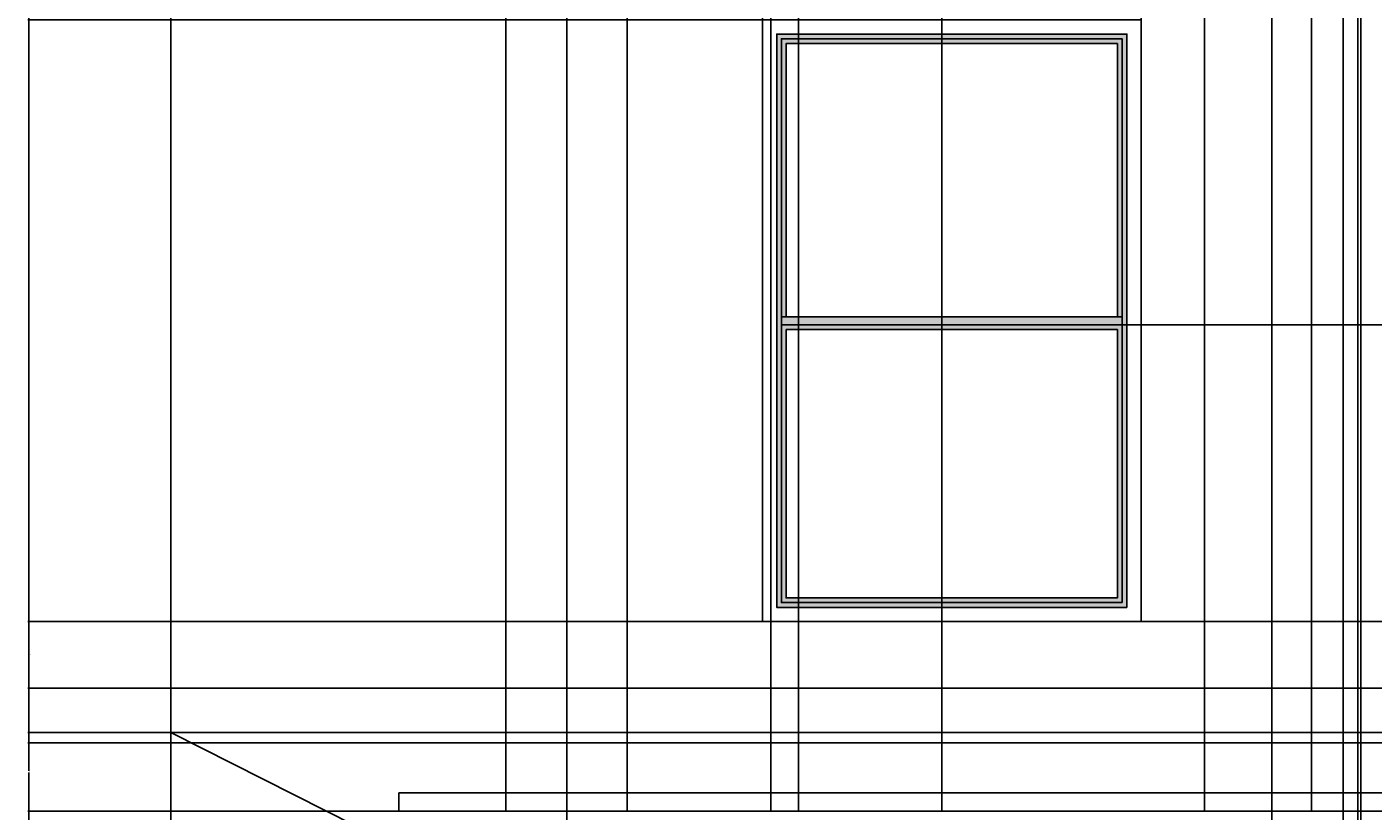
# Model space of a CAD drawing. Units: millimetres. Extents: x 171 to 1599, y 973 to 1509.
# Tile 3 of 7: x 951 to 1235, y 1178 to 1343. Entities that reach past the tile are written whole.
import ezdxf

# ---------------------------------------------------------------- set-up
doc = ezdxf.new("R2010")
doc.units = ezdxf.units.MM
for name, color, linetype, lineweight in [('A-ANNO-DIMS', 2, 'Continuous', 18), ('A-ELEV', 7, 'Continuous', 25), ('A-ELEV-FILL', 252, 'Continuous', 13)]:
    doc.layers.add(name, color=color, linetype=linetype, lineweight=lineweight)
doc.styles.get("Standard").update_dxf_attribs({"font": 'arial.ttf'})
doc.dimstyles.get("Standard").update_dxf_attribs({"dimtxt": 0.18, "dimasz": 0.18, "dimexe": 0.18, "dimexo": 0.0625, "dimgap": 0.09, "dimtad": 0, "dimtih": 1, "dimtoh": 1, "dimdec": 1, "dimzin": 0, "dimdsep": 46, "dimlunit": 3, "dimtxsty": 'Standard', "dimcen": 0.09, "dimadec": 0, "dimazin": 0, "dimtfac": 1, "dimtdec": 1, "dimtofl": 0, "dimtmove": 0, "dimatfit": 3, "dimfxl": 1, "dimtolj": 1, "dimtzin": 0, "dimarcsym": 0})

# ---------------------------------------------------------------- blocks, each defined once
blk = doc.blocks.new('*D1')
at = {"layer": 'A-ANNO-DIMS', "color": 0, "lineweight": -2, "transparency": 16777216}
for p, q in [((980.93, 1194.55), (980.93, 1508.31)), ((981.11, 1508.13), (1274.61, 1508.13)), ((1568.85, 1508.13), (1275.36, 1508.13)), ((1569.03, 1215.31), (1569.03, 1508.31))]:
    blk.add_line(p, q, dxfattribs=at)
at = {"layer": 'A-ANNO-DIMS', "color": 0, "transparency": 16777216}
for points in [[(981.11, 1508.16), (981.11, 1508.1), (980.93, 1508.13)], [(1568.85, 1508.16), (1568.85, 1508.1), (1569.03, 1508.13)]]:
    blk.add_solid(points, dxfattribs=at)
at = {"layer": 'Defpoints', "color": 0, "transparency": 16777216}
for p in [(1569.03, 1508.13), (1569.03, 1215.25), (980.93, 1194.49)]:
    blk.add_point(p, dxfattribs=at)
at = {"layer": 'A-ANNO-DIMS', "color": 0, "transparency": 16777216, "insert": (1274.98, 1508.13), "char_height": 0.18, "attachment_point": 5}
blk.add_mtext('\\A1;588.1', dxfattribs=at)
blk = doc.blocks.new('*D2')
at = {"layer": 'A-ANNO-DIMS', "color": 0, "lineweight": -2, "transparency": 16777216}
for p, q in [((1043.70287, 1478.130098), (1599.212656, 1478.130098)), ((1599.032656, 1477.950098), (1599.032656, 1240.959874)), ((1599.032656, 1003.60965), (1599.032656, 1240.599874)), ((1348.449149, 1003.42965), (1599.212656, 1003.42965))]:
    blk.add_line(p, q, dxfattribs=at)
at = {"layer": 'A-ANNO-DIMS', "color": 0, "transparency": 16777216}
for points in [[(1599.002656, 1477.950098), (1599.062656, 1477.950098), (1599.032656, 1478.130098)], [(1599.002656, 1003.60965), (1599.062656, 1003.60965), (1599.032656, 1003.42965)]]:
    blk.add_solid(points, dxfattribs=at)
at = {"layer": 'Defpoints', "color": 0, "transparency": 16777216}
for p in [(1043.64037, 1478.130098), (1599.032656, 1478.130098), (1348.386649, 1003.42965)]:
    blk.add_point(p, dxfattribs=at)
at = {"layer": 'A-ANNO-DIMS', "color": 0, "transparency": 16777216, "insert": (1599.032656, 1240.779874), "char_height": 0.18, "attachment_point": 5}
blk.add_mtext('\\A1;474.7', dxfattribs=at)
blk = doc.blocks.new('*D13')
at = {"layer": 'A-ANNO-DIMS', "color": 0, "lineweight": -2, "transparency": 16777216}
for p, q in [((1029, 1177.87), (950.75, 1177.87)), ((950.93, 1177.69), (950.93, 1108.74)), ((950.93, 1039.43), (950.93, 1108.38)), ((1029, 1039.25), (950.75, 1039.25))]:
    blk.add_line(p, q, dxfattribs=at)
at = {"layer": 'A-ANNO-DIMS', "color": 0, "transparency": 16777216}
for points in [[(950.9, 1177.69), (950.96, 1177.69), (950.93, 1177.87)], [(950.9, 1039.43), (950.96, 1039.43), (950.93, 1039.25)]]:
    blk.add_solid(points, dxfattribs=at)
at = {"layer": 'Defpoints', "color": 0, "transparency": 16777216}
for p in [(950.93, 1177.87), (1029.07, 1177.87), (1029.07, 1039.25)]:
    blk.add_point(p, dxfattribs=at)
at = {"layer": 'A-ANNO-DIMS', "color": 0, "transparency": 16777216, "insert": (950.93, 1108.56), "char_height": 0.18, "attachment_point": 5}
blk.add_mtext('\\A1;138.62', dxfattribs=at)
blk = doc.blocks.new('*D14')
at = {"layer": 'A-ANNO-DIMS', "color": 0, "lineweight": -2, "transparency": 16777216}
for p, q in [((980.87, 1194.49), (950.75, 1194.49)), ((950.93, 1194.31), (950.93, 1186.36)), ((950.93, 1178.05), (950.93, 1186)), ((1029, 1177.87), (950.75, 1177.87))]:
    blk.add_line(p, q, dxfattribs=at)
at = {"layer": 'A-ANNO-DIMS', "color": 0, "transparency": 16777216}
for points in [[(950.9, 1194.31), (950.96, 1194.31), (950.93, 1194.49)], [(950.9, 1178.05), (950.96, 1178.05), (950.93, 1177.87)]]:
    blk.add_solid(points, dxfattribs=at)
at = {"layer": 'Defpoints', "color": 0, "transparency": 16777216}
for p in [(950.93, 1194.49), (980.93, 1194.49), (1029.07, 1177.87)]:
    blk.add_point(p, dxfattribs=at)
at = {"layer": 'A-ANNO-DIMS', "color": 0, "transparency": 16777216, "insert": (950.93, 1186.18), "char_height": 0.18, "attachment_point": 5}
blk.add_mtext('\\A1;16.616', dxfattribs=at)
blk = doc.blocks.new('*D15')
at = {"layer": 'A-ANNO-DIMS', "color": 0, "lineweight": -2, "transparency": 16777216}
for p, q in [((980.87, 1203.79), (950.75, 1203.79)), ((950.93, 1203.61), (950.93, 1199.32)), ((950.93, 1194.67), (950.93, 1198.96)), ((980.87, 1194.49), (950.75, 1194.49))]:
    blk.add_line(p, q, dxfattribs=at)
at = {"layer": 'A-ANNO-DIMS', "color": 0, "transparency": 16777216}
for points in [[(950.9, 1203.61), (950.96, 1203.61), (950.93, 1203.79)], [(950.9, 1194.67), (950.96, 1194.67), (950.93, 1194.49)]]:
    blk.add_solid(points, dxfattribs=at)
at = {"layer": 'Defpoints', "color": 0, "transparency": 16777216}
for p in [(950.93, 1203.79), (980.93, 1203.79), (980.93, 1194.49)]:
    blk.add_point(p, dxfattribs=at)
at = {"layer": 'A-ANNO-DIMS', "color": 0, "transparency": 16777216, "insert": (950.93, 1199.14), "char_height": 0.18, "attachment_point": 5}
blk.add_mtext('\\A1;9.306', dxfattribs=at)
blk = doc.blocks.new('*D16')
at = {"layer": 'A-ANNO-DIMS', "color": 0, "lineweight": -2, "transparency": 16777216}
for p, q in [((1105.76, 1217.87), (950.75, 1217.87)), ((950.93, 1217.69), (950.93, 1211.01)), ((950.93, 1203.97), (950.93, 1210.65)), ((980.87, 1203.79), (950.75, 1203.79))]:
    blk.add_line(p, q, dxfattribs=at)
at = {"layer": 'A-ANNO-DIMS', "color": 0, "transparency": 16777216}
for points in [[(950.9, 1217.69), (950.96, 1217.69), (950.93, 1217.87)], [(950.9, 1203.97), (950.96, 1203.97), (950.93, 1203.79)]]:
    blk.add_solid(points, dxfattribs=at)
at = {"layer": 'Defpoints', "color": 0, "transparency": 16777216}
for p in [(950.93, 1217.87), (1105.82, 1217.87), (980.93, 1203.79)]:
    blk.add_point(p, dxfattribs=at)
at = {"layer": 'A-ANNO-DIMS', "color": 0, "transparency": 16777216, "insert": (950.93, 1210.83), "char_height": 0.18, "attachment_point": 5}
blk.add_mtext('\\A1;14.073', dxfattribs=at)
blk = doc.blocks.new('*D17')
at = {"layer": 'A-ANNO-DIMS', "color": 0, "lineweight": -2, "transparency": 16777216}
for p, q in [((1105.76, 1344.87), (950.75, 1344.87)), ((950.93, 1344.69), (950.93, 1281.55)), ((950.93, 1218.05), (950.93, 1281.19)), ((1105.76, 1217.87), (950.75, 1217.87))]:
    blk.add_line(p, q, dxfattribs=at)
at = {"layer": 'A-ANNO-DIMS', "color": 0, "transparency": 16777216}
for points in [[(950.9, 1344.69), (950.96, 1344.69), (950.93, 1344.87)], [(950.9, 1218.05), (950.96, 1218.05), (950.93, 1217.87)]]:
    blk.add_solid(points, dxfattribs=at)
at = {"layer": 'Defpoints', "color": 0, "transparency": 16777216}
for p in [(950.93, 1344.87), (1105.82, 1344.87), (1105.82, 1217.87)]:
    blk.add_point(p, dxfattribs=at)
at = {"layer": 'A-ANNO-DIMS', "color": 0, "transparency": 16777216, "insert": (950.93, 1281.37), "char_height": 0.18, "attachment_point": 5}
blk.add_mtext('\\A1;127', dxfattribs=at)
blk = doc.blocks.new('*D38')
at = {"layer": 'A-ANNO-DIMS', "color": 0, "lineweight": -2, "transparency": 16777216}
for p, q in [((980.93, 1203.86), (980.93, 1508.31)), ((981.11, 1508.13), (991.19, 1508.13)), ((1002.21, 1508.13), (992.12, 1508.13)), ((1002.39, 1430.6), (1002.39, 1508.31))]:
    blk.add_line(p, q, dxfattribs=at)
at = {"layer": 'A-ANNO-DIMS', "color": 0, "transparency": 16777216}
for points in [[(981.11, 1508.16), (981.11, 1508.1), (980.93, 1508.13)], [(1002.21, 1508.16), (1002.21, 1508.1), (1002.39, 1508.13)]]:
    blk.add_solid(points, dxfattribs=at)
at = {"layer": 'Defpoints', "color": 0, "transparency": 16777216}
for p in [(1002.39, 1508.13), (1002.39, 1430.53), (980.93, 1203.79)]:
    blk.add_point(p, dxfattribs=at)
at = {"layer": 'A-ANNO-DIMS', "color": 0, "transparency": 16777216, "insert": (991.66, 1508.13), "char_height": 0.18, "attachment_point": 5}
blk.add_mtext('\\A1;21.455', dxfattribs=at)
blk = doc.blocks.new('*D42')
at = {"layer": 'A-ANNO-DIMS', "color": 0, "lineweight": -2, "transparency": 16777216}
for p, q in [((1192.02, 1419.99), (1192.02, 1508.31)), ((1192.2, 1508.13), (1378.72, 1508.13)), ((1566.18, 1508.13), (1379.65, 1508.13)), ((1566.36, 1203.87), (1566.36, 1508.31))]:
    blk.add_line(p, q, dxfattribs=at)
at = {"layer": 'A-ANNO-DIMS', "color": 0, "transparency": 16777216}
for points in [[(1192.2, 1508.16), (1192.2, 1508.1), (1192.02, 1508.13)], [(1566.18, 1508.16), (1566.18, 1508.1), (1566.36, 1508.13)]]:
    blk.add_solid(points, dxfattribs=at)
at = {"layer": 'Defpoints', "color": 0, "transparency": 16777216}
for p in [(1566.36, 1508.13), (1192.02, 1419.93), (1566.36, 1203.8)]:
    blk.add_point(p, dxfattribs=at)
at = {"layer": 'A-ANNO-DIMS', "color": 0, "transparency": 16777216, "insert": (1379.19, 1508.13), "char_height": 0.18, "attachment_point": 5}
blk.add_mtext('\\A1;374.34', dxfattribs=at)
blk = doc.blocks.new('*D47')
at = {"layer": 'A-ANNO-DIMS', "color": 0, "lineweight": -2, "transparency": 16777216}
for p, q in [((1192.08, 1419.93), (1599.21, 1419.93)), ((1599.03, 1419.75), (1599.03, 1312.05)), ((1599.03, 1203.98), (1599.03, 1311.68)), ((1566.42, 1203.8), (1599.21, 1203.8))]:
    blk.add_line(p, q, dxfattribs=at)
at = {"layer": 'A-ANNO-DIMS', "color": 0, "transparency": 16777216}
for points in [[(1599, 1419.75), (1599.06, 1419.75), (1599.03, 1419.93)], [(1599, 1203.98), (1599.06, 1203.98), (1599.03, 1203.8)]]:
    blk.add_solid(points, dxfattribs=at)
at = {"layer": 'Defpoints', "color": 0, "transparency": 16777216}
for p in [(1192.02, 1419.93), (1566.36, 1203.8), (1599.03, 1203.8)]:
    blk.add_point(p, dxfattribs=at)
at = {"layer": 'A-ANNO-DIMS', "color": 0, "transparency": 16777216, "insert": (1599.03, 1311.87), "char_height": 0.18, "attachment_point": 5}
blk.add_mtext('\\A1;216.13', dxfattribs=at)
blk = doc.blocks.new('*D49')
at = {"layer": 'A-ANNO-DIMS', "color": 0, "lineweight": -2, "transparency": 16777216}
for p, q in [((1064.5, 1203.86), (1064.5, 1508.31)), ((1064.68, 1508.13), (1084.78, 1508.13)), ((1105.64, 1508.13), (1085.54, 1508.13)), ((1105.82, 1344.93), (1105.82, 1508.31))]:
    blk.add_line(p, q, dxfattribs=at)
at = {"layer": 'A-ANNO-DIMS', "color": 0, "transparency": 16777216}
for points in [[(1064.68, 1508.16), (1064.68, 1508.1), (1064.5, 1508.13)], [(1105.64, 1508.16), (1105.64, 1508.1), (1105.82, 1508.13)]]:
    blk.add_solid(points, dxfattribs=at)
at = {"layer": 'Defpoints', "color": 0, "transparency": 16777216}
for p in [(1105.82, 1508.13), (1105.82, 1344.87), (1064.5, 1203.79)]:
    blk.add_point(p, dxfattribs=at)
at = {"layer": 'A-ANNO-DIMS', "color": 0, "transparency": 16777216, "insert": (1085.16, 1508.13), "char_height": 0.18, "attachment_point": 5}
blk.add_mtext('\\A1;41.31', dxfattribs=at)
blk = doc.blocks.new('*D51')
at = {"layer": 'A-ANNO-DIMS', "color": 0, "lineweight": -2, "transparency": 16777216}
for p, q in [((1185.73, 1344.93), (1185.73, 1508.31)), ((1185.91, 1508.13), (1199.08, 1508.13)), ((1213.17, 1508.13), (1200.01, 1508.13)), ((1213.35, 1203.86), (1213.35, 1508.31))]:
    blk.add_line(p, q, dxfattribs=at)
at = {"layer": 'A-ANNO-DIMS', "color": 0, "transparency": 16777216}
for points in [[(1185.91, 1508.16), (1185.91, 1508.1), (1185.73, 1508.13)], [(1213.17, 1508.16), (1213.17, 1508.1), (1213.35, 1508.13)]]:
    blk.add_solid(points, dxfattribs=at)
at = {"layer": 'Defpoints', "color": 0, "transparency": 16777216}
for p in [(1213.35, 1508.13), (1185.73, 1344.87), (1213.35, 1203.79)]:
    blk.add_point(p, dxfattribs=at)
at = {"layer": 'A-ANNO-DIMS', "color": 0, "transparency": 16777216, "insert": (1199.54, 1508.13), "char_height": 0.18, "attachment_point": 5}
blk.add_mtext('\\A1;27.614', dxfattribs=at)
blk = doc.blocks.new('*D52')
at = {"layer": 'A-ANNO-DIMS', "color": 0, "lineweight": -2, "transparency": 16777216}
for p, q in [((1064.5, 1203.73), (1064.5, 973.25)), ((980.93, 1194.43), (980.93, 973.25)), ((981.11, 973.43), (1022.32, 973.43)), ((1064.32, 973.43), (1023.11, 973.43))]:
    blk.add_line(p, q, dxfattribs=at)
at = {"layer": 'A-ANNO-DIMS', "color": 0, "transparency": 16777216}
for points in [[(981.11, 973.46), (981.11, 973.4), (980.93, 973.43)], [(1064.32, 973.46), (1064.32, 973.4), (1064.5, 973.43)]]:
    blk.add_solid(points, dxfattribs=at)
at = {"layer": 'Defpoints', "color": 0, "transparency": 16777216}
for p in [(1064.5, 1203.79), (980.93, 1194.49), (1064.5, 973.43)]:
    blk.add_point(p, dxfattribs=at)
at = {"layer": 'A-ANNO-DIMS', "color": 0, "transparency": 16777216, "insert": (1022.72, 973.43), "char_height": 0.18, "attachment_point": 5}
blk.add_mtext('\\A1;83.57', dxfattribs=at)
blk = doc.blocks.new('*D53')
at = {"layer": 'A-ANNO-DIMS', "color": 0, "lineweight": -2, "transparency": 16777216}
for p, q in [((1213.35, 1203.73), (1213.35, 973.25)), ((1232.1, 1203.73), (1232.1, 973.25)), ((1213.53, 973.43), (1222.34, 973.43)), ((1231.92, 973.43), (1223.11, 973.43))]:
    blk.add_line(p, q, dxfattribs=at)
at = {"layer": 'A-ANNO-DIMS', "color": 0, "transparency": 16777216}
for points in [[(1213.53, 973.46), (1213.53, 973.4), (1213.35, 973.43)], [(1231.92, 973.46), (1231.92, 973.4), (1232.1, 973.43)]]:
    blk.add_solid(points, dxfattribs=at)
at = {"layer": 'Defpoints', "color": 0, "transparency": 16777216}
for p in [(1213.35, 1203.79), (1232.1, 1203.79), (1232.1, 973.43)]:
    blk.add_point(p, dxfattribs=at)
at = {"layer": 'A-ANNO-DIMS', "color": 0, "transparency": 16777216, "insert": (1222.72, 973.43), "char_height": 0.18, "attachment_point": 5}
blk.add_mtext('\\A1;18.75', dxfattribs=at)
blk = doc.blocks.new('*D54')
at = {"layer": 'A-ANNO-DIMS', "color": 0, "lineweight": -2, "transparency": 16777216}
for p, q in [((1232.1, 1203.73), (1232.1, 973.25)), ((1320.32, 1192.2), (1320.32, 973.25)), ((1232.28, 973.43), (1275.82, 973.43)), ((1320.14, 973.43), (1276.6, 973.43))]:
    blk.add_line(p, q, dxfattribs=at)
at = {"layer": 'A-ANNO-DIMS', "color": 0, "transparency": 16777216}
for points in [[(1232.28, 973.46), (1232.28, 973.4), (1232.1, 973.43)], [(1320.14, 973.46), (1320.14, 973.4), (1320.32, 973.43)]]:
    blk.add_solid(points, dxfattribs=at)
at = {"layer": 'Defpoints', "color": 0, "transparency": 16777216}
for p in [(1232.1, 1203.79), (1320.32, 1192.27), (1320.32, 973.43)]:
    blk.add_point(p, dxfattribs=at)
at = {"layer": 'A-ANNO-DIMS', "color": 0, "transparency": 16777216, "insert": (1276.21, 973.43), "char_height": 0.18, "attachment_point": 5}
blk.add_mtext('\\A1;88.22', dxfattribs=at)
blk = doc.blocks.new('*D61')
at = {"layer": 'A-ANNO-DIMS', "color": 0, "lineweight": -2, "transparency": 16777216}
for p, q in [((1320.26, 1345.85), (950.75, 1345.85)), ((950.93, 1345.67), (950.93, 1269.24)), ((950.93, 1192.45), (950.93, 1268.88)), ((1320.26, 1192.27), (950.75, 1192.27))]:
    blk.add_line(p, q, dxfattribs=at)
at = {"layer": 'A-ANNO-DIMS', "color": 0, "transparency": 16777216}
for points in [[(950.9, 1345.67), (950.96, 1345.67), (950.93, 1345.85)], [(950.9, 1192.45), (950.96, 1192.45), (950.93, 1192.27)]]:
    blk.add_solid(points, dxfattribs=at)
at = {"layer": 'Defpoints', "color": 0, "transparency": 16777216}
for p in [(950.93, 1345.85), (1320.32, 1345.85), (1320.32, 1192.27)]:
    blk.add_point(p, dxfattribs=at)
at = {"layer": 'A-ANNO-DIMS', "color": 0, "transparency": 16777216, "insert": (950.93, 1269.06), "char_height": 0.18, "attachment_point": 5}
blk.add_mtext('\\A1;153.59', dxfattribs=at)
blk = doc.blocks.new('*D63')
at = {"layer": 'A-ANNO-DIMS', "color": 0, "lineweight": -2, "transparency": 16777216}
for p, q in [((1181.8, 1280.52), (1599.21, 1280.52)), ((1599.03, 1280.34), (1599.03, 1249.38)), ((1599.03, 1218.05), (1599.03, 1249.01)), ((1185.8, 1217.87), (1599.21, 1217.87))]:
    blk.add_line(p, q, dxfattribs=at)
at = {"layer": 'A-ANNO-DIMS', "color": 0, "transparency": 16777216}
for points in [[(1599, 1280.34), (1599.06, 1280.34), (1599.03, 1280.52)], [(1599, 1218.05), (1599.06, 1218.05), (1599.03, 1217.87)]]:
    blk.add_solid(points, dxfattribs=at)
at = {"layer": 'Defpoints', "color": 0, "transparency": 16777216}
for p in [(1181.73, 1280.52), (1599.03, 1280.52), (1185.73, 1217.87)]:
    blk.add_point(p, dxfattribs=at)
at = {"layer": 'A-ANNO-DIMS', "color": 0, "transparency": 16777216, "insert": (1599.03, 1249.2), "char_height": 0.18, "attachment_point": 5}
blk.add_mtext('\\A1;62.66', dxfattribs=at)
blk = doc.blocks.new('*D64')
at = {"layer": 'A-ANNO-DIMS', "color": 0, "lineweight": -2, "transparency": 16777216}
for p, q in [((1051.62, 1177.93), (1051.62, 1508.31)), ((1051.8, 1508.13), (1057.61, 1508.13)), ((1064.32, 1508.13), (1058.52, 1508.13)), ((1064.5, 1177.93), (1064.5, 1508.31))]:
    blk.add_line(p, q, dxfattribs=at)
at = {"layer": 'A-ANNO-DIMS', "color": 0, "transparency": 16777216}
for points in [[(1051.8, 1508.16), (1051.8, 1508.1), (1051.62, 1508.13)], [(1064.32, 1508.16), (1064.32, 1508.1), (1064.5, 1508.13)]]:
    blk.add_solid(points, dxfattribs=at)
at = {"layer": 'Defpoints', "color": 0, "transparency": 16777216}
for p in [(1064.5, 1508.13), (1051.62, 1177.87), (1064.5, 1177.87)]:
    blk.add_point(p, dxfattribs=at)
at = {"layer": 'A-ANNO-DIMS', "color": 0, "transparency": 16777216, "insert": (1058.06, 1508.13), "char_height": 0.18, "attachment_point": 5}
blk.add_mtext('\\A1;12.882', dxfattribs=at)
blk = doc.blocks.new('*D65')
at = {"layer": 'A-ANNO-DIMS', "color": 0, "lineweight": -2, "transparency": 16777216}
for p, q in [((1064.5, 1177.93), (1064.5, 1508.31)), ((1064.68, 1508.13), (1070.43, 1508.13)), ((1077.09, 1508.13), (1071.34, 1508.13)), ((1077.27, 1177.93), (1077.27, 1508.31))]:
    blk.add_line(p, q, dxfattribs=at)
at = {"layer": 'A-ANNO-DIMS', "color": 0, "transparency": 16777216}
for points in [[(1064.68, 1508.16), (1064.68, 1508.1), (1064.5, 1508.13)], [(1077.09, 1508.16), (1077.09, 1508.1), (1077.27, 1508.13)]]:
    blk.add_solid(points, dxfattribs=at)
at = {"layer": 'Defpoints', "color": 0, "transparency": 16777216}
for p in [(1077.27, 1508.13), (1064.5, 1177.87), (1077.27, 1177.87)]:
    blk.add_point(p, dxfattribs=at)
at = {"layer": 'A-ANNO-DIMS', "color": 0, "transparency": 16777216, "insert": (1070.89, 1508.13), "char_height": 0.18, "attachment_point": 5}
blk.add_mtext('\\A1;12.767', dxfattribs=at)
blk = doc.blocks.new('*D66')
at = {"layer": 'A-ANNO-DIMS', "color": 0, "lineweight": -2, "transparency": 16777216}
for p, q in [((1077.27, 1177.93), (1077.27, 1508.31)), ((1077.45, 1508.13), (1092.02, 1508.13)), ((1107.38, 1508.13), (1092.81, 1508.13)), ((1107.56, 1177.93), (1107.56, 1508.31))]:
    blk.add_line(p, q, dxfattribs=at)
at = {"layer": 'A-ANNO-DIMS', "color": 0, "transparency": 16777216}
for points in [[(1077.45, 1508.16), (1077.45, 1508.1), (1077.27, 1508.13)], [(1107.38, 1508.16), (1107.38, 1508.1), (1107.56, 1508.13)]]:
    blk.add_solid(points, dxfattribs=at)
at = {"layer": 'Defpoints', "color": 0, "transparency": 16777216}
for p in [(1107.56, 1508.13), (1077.27, 1177.87), (1107.56, 1177.87)]:
    blk.add_point(p, dxfattribs=at)
at = {"layer": 'A-ANNO-DIMS', "color": 0, "transparency": 16777216, "insert": (1092.42, 1508.13), "char_height": 0.18, "attachment_point": 5}
blk.add_mtext('\\A1;30.29', dxfattribs=at)
blk = doc.blocks.new('*D67')
at = {"layer": 'A-ANNO-DIMS', "color": 0, "lineweight": -2, "transparency": 16777216}
for p, q in [((1107.56, 1177.93), (1107.56, 1508.31)), ((1107.74, 1508.13), (1110.09, 1508.13)), ((1113.23, 1508.13), (1110.88, 1508.13)), ((1113.41, 1177.93), (1113.41, 1508.31))]:
    blk.add_line(p, q, dxfattribs=at)
at = {"layer": 'A-ANNO-DIMS', "color": 0, "transparency": 16777216}
for points in [[(1107.74, 1508.16), (1107.74, 1508.1), (1107.56, 1508.13)], [(1113.23, 1508.16), (1113.23, 1508.1), (1113.41, 1508.13)]]:
    blk.add_solid(points, dxfattribs=at)
at = {"layer": 'Defpoints', "color": 0, "transparency": 16777216}
for p in [(1113.41, 1508.13), (1107.56, 1177.87), (1113.41, 1177.87)]:
    blk.add_point(p, dxfattribs=at)
at = {"layer": 'A-ANNO-DIMS', "color": 0, "transparency": 16777216, "insert": (1110.49, 1508.13), "char_height": 0.18, "attachment_point": 5}
blk.add_mtext('\\A1;5.847', dxfattribs=at)
blk = doc.blocks.new('*D68')
at = {"layer": 'A-ANNO-DIMS', "color": 0, "lineweight": -2, "transparency": 16777216}
for p, q in [((1113.41, 1177.93), (1113.41, 1508.31)), ((1113.59, 1508.13), (1128.16, 1508.13)), ((1143.52, 1508.13), (1128.95, 1508.13)), ((1143.7, 1177.93), (1143.7, 1508.31))]:
    blk.add_line(p, q, dxfattribs=at)
at = {"layer": 'A-ANNO-DIMS', "color": 0, "transparency": 16777216}
for points in [[(1113.59, 1508.16), (1113.59, 1508.1), (1113.41, 1508.13)], [(1143.52, 1508.16), (1143.52, 1508.1), (1143.7, 1508.13)]]:
    blk.add_solid(points, dxfattribs=at)
at = {"layer": 'Defpoints', "color": 0, "transparency": 16777216}
for p in [(1143.7, 1508.13), (1113.41, 1177.87), (1143.7, 1177.87)]:
    blk.add_point(p, dxfattribs=at)
at = {"layer": 'A-ANNO-DIMS', "color": 0, "transparency": 16777216, "insert": (1128.55, 1508.13), "char_height": 0.18, "attachment_point": 5}
blk.add_mtext('\\A1;30.29', dxfattribs=at)
blk = doc.blocks.new('*D69')
at = {"layer": 'A-ANNO-DIMS', "color": 0, "lineweight": -2, "transparency": 16777216}
for p, q in [((1143.7, 1177.93), (1143.7, 1508.31)), ((1143.88, 1508.13), (1171.03, 1508.13)), ((1198.93, 1508.13), (1171.78, 1508.13)), ((1199.11, 1177.93), (1199.11, 1508.31))]:
    blk.add_line(p, q, dxfattribs=at)
at = {"layer": 'A-ANNO-DIMS', "color": 0, "transparency": 16777216}
for points in [[(1143.88, 1508.16), (1143.88, 1508.1), (1143.7, 1508.13)], [(1198.93, 1508.16), (1198.93, 1508.1), (1199.11, 1508.13)]]:
    blk.add_solid(points, dxfattribs=at)
at = {"layer": 'Defpoints', "color": 0, "transparency": 16777216}
for p in [(1199.11, 1508.13), (1143.7, 1177.87), (1199.11, 1177.87)]:
    blk.add_point(p, dxfattribs=at)
at = {"layer": 'A-ANNO-DIMS', "color": 0, "transparency": 16777216, "insert": (1171.4, 1508.13), "char_height": 0.18, "attachment_point": 5}
blk.add_mtext('\\A1;55.41', dxfattribs=at)
blk = doc.blocks.new('*D70')
at = {"layer": 'A-ANNO-DIMS', "color": 0, "lineweight": -2, "transparency": 16777216}
for p, q in [((1199.11, 1177.93), (1199.11, 1508.31)), ((1199.29, 1508.13), (1210.04, 1508.13)), ((1221.54, 1508.13), (1210.79, 1508.13)), ((1221.72, 1177.93), (1221.72, 1508.31))]:
    blk.add_line(p, q, dxfattribs=at)
at = {"layer": 'A-ANNO-DIMS', "color": 0, "transparency": 16777216}
for points in [[(1199.29, 1508.16), (1199.29, 1508.1), (1199.11, 1508.13)], [(1221.54, 1508.16), (1221.54, 1508.1), (1221.72, 1508.13)]]:
    blk.add_solid(points, dxfattribs=at)
at = {"layer": 'Defpoints', "color": 0, "transparency": 16777216}
for p in [(1221.72, 1508.13), (1199.11, 1177.87), (1221.72, 1177.87)]:
    blk.add_point(p, dxfattribs=at)
at = {"layer": 'A-ANNO-DIMS', "color": 0, "transparency": 16777216, "insert": (1210.41, 1508.13), "char_height": 0.18, "attachment_point": 5}
blk.add_mtext('\\A1;22.61', dxfattribs=at)
blk = doc.blocks.new('*D71')
at = {"layer": 'A-ANNO-DIMS', "color": 0, "lineweight": -2, "transparency": 16777216}
for p, q in [((1221.72, 1177.93), (1221.72, 1508.31)), ((1221.9, 1508.13), (1224.73, 1508.13)), ((1228.22, 1508.13), (1225.38, 1508.13)), ((1228.4, 1114.32), (1228.4, 1508.31))]:
    blk.add_line(p, q, dxfattribs=at)
at = {"layer": 'A-ANNO-DIMS', "color": 0, "transparency": 16777216}
for points in [[(1221.9, 1508.16), (1221.9, 1508.1), (1221.72, 1508.13)], [(1228.22, 1508.16), (1228.22, 1508.1), (1228.4, 1508.13)]]:
    blk.add_solid(points, dxfattribs=at)
at = {"layer": 'Defpoints', "color": 0, "transparency": 16777216}
for p in [(1228.4, 1508.13), (1221.72, 1177.87), (1228.4, 1114.25)]:
    blk.add_point(p, dxfattribs=at)
at = {"layer": 'A-ANNO-DIMS', "color": 0, "transparency": 16777216, "insert": (1225.06, 1508.13), "char_height": 0.18, "attachment_point": 5}
blk.add_mtext('\\A1;6.68', dxfattribs=at)
blk = doc.blocks.new('*D72')
at = {"layer": 'A-ANNO-DIMS', "color": 0, "lineweight": -2, "transparency": 16777216}
for p, q in [((1228.4, 1114.32), (1228.4, 1508.31)), ((1228.58, 1508.13), (1229.61, 1508.13)), ((1231.28, 1508.13), (1230.25, 1508.13)), ((1231.46, 1114.32), (1231.46, 1508.31))]:
    blk.add_line(p, q, dxfattribs=at)
at = {"layer": 'A-ANNO-DIMS', "color": 0, "transparency": 16777216}
for points in [[(1228.58, 1508.16), (1228.58, 1508.1), (1228.4, 1508.13)], [(1231.28, 1508.16), (1231.28, 1508.1), (1231.46, 1508.13)]]:
    blk.add_solid(points, dxfattribs=at)
at = {"layer": 'Defpoints', "color": 0, "transparency": 16777216}
for p in [(1231.46, 1508.13), (1228.4, 1114.25), (1231.46, 1114.25)]:
    blk.add_point(p, dxfattribs=at)
at = {"layer": 'A-ANNO-DIMS', "color": 0, "transparency": 16777216, "insert": (1229.93, 1508.13), "char_height": 0.18, "attachment_point": 5}
blk.add_mtext('\\A1;3.06', dxfattribs=at)
blk = doc.blocks.new('*D73')
at = {"layer": 'A-ANNO-DIMS', "color": 0, "lineweight": -2, "transparency": 16777216}
for p, q in [((1231.46, 1114.32), (1231.46, 1508.31)), ((1231.64, 1508.13), (1234.06, 1508.13)), ((1237.13, 1508.13), (1234.71, 1508.13)), ((1237.31, 1162.35), (1237.31, 1508.31))]:
    blk.add_line(p, q, dxfattribs=at)
at = {"layer": 'A-ANNO-DIMS', "color": 0, "transparency": 16777216}
for points in [[(1231.64, 1508.16), (1231.64, 1508.1), (1231.46, 1508.13)], [(1237.13, 1508.16), (1237.13, 1508.1), (1237.31, 1508.13)]]:
    blk.add_solid(points, dxfattribs=at)
at = {"layer": 'Defpoints', "color": 0, "transparency": 16777216}
for p in [(1237.31, 1508.13), (1237.31, 1162.29), (1231.46, 1114.25)]:
    blk.add_point(p, dxfattribs=at)
at = {"layer": 'A-ANNO-DIMS', "color": 0, "transparency": 16777216, "insert": (1234.38, 1508.13), "char_height": 0.18, "attachment_point": 5}
blk.add_mtext('\\A1;5.85', dxfattribs=at)
blk = doc.blocks.new('*D83')
at = {"layer": 'A-ANNO-DIMS', "color": 0, "lineweight": -2, "transparency": 16777216}
for p, q in [((1143.64, 1177.87), (950.75, 1177.87)), ((950.93, 1177.69), (950.93, 1130.23)), ((950.93, 1082.41), (950.93, 1129.87)), ((1143.64, 1082.23), (950.75, 1082.23))]:
    blk.add_line(p, q, dxfattribs=at)
at = {"layer": 'A-ANNO-DIMS', "color": 0, "transparency": 16777216}
for points in [[(950.9, 1177.69), (950.96, 1177.69), (950.93, 1177.87)], [(950.9, 1082.41), (950.96, 1082.41), (950.93, 1082.23)]]:
    blk.add_solid(points, dxfattribs=at)
at = {"layer": 'Defpoints', "color": 0, "transparency": 16777216}
for p in [(950.93, 1177.87), (1143.7, 1177.87), (1143.7, 1082.23)]:
    blk.add_point(p, dxfattribs=at)
at = {"layer": 'A-ANNO-DIMS', "color": 0, "transparency": 16777216, "insert": (950.93, 1130.05), "char_height": 0.18, "attachment_point": 5}
blk.add_mtext('\\A1;95.64', dxfattribs=at)

msp = doc.modelspace()

# ---------------------------------------------------------------- hatches: boundary and pattern name
at = {"layer": 'A-ELEV-FILL'}
h = msp.add_hatch(color=256, dxfattribs=at)
h.dxf.hatch_style = 1
h.paths.add_polyline_path([(1182.7346, 1341.8717), (1108.8176, 1341.8717), (1108.8176, 1220.867), (1182.7346, 1220.867)])
h.paths.add_polyline_path([(1181.7346, 1221.867), (1109.8176, 1221.867), (1109.8176, 1340.8717), (1181.7346, 1340.8717)], flags=16)
h.paths.add_polyline_path([(1180.7346, 1339.8717), (1180.7346, 1282.2145), (1181.7346, 1282.2145), (1181.7346, 1280.5242), (1109.8176, 1280.5242), (1109.8176, 1282.2145), (1110.8176, 1282.2145), (1110.8176, 1339.8717)], flags=0)
h.paths.add_polyline_path([(1180.7346, 1279.5242), (1180.7346, 1222.867), (1110.8176, 1222.867), (1110.8176, 1279.5242)], flags=0)
h.paths.add_polyline_path([(1387.6984, 1172.7441), (1384.4743, 1172.7441), (1384.4743, 1086.2327), (1387.6984, 1086.2327)])
h = msp.add_hatch(color=256, dxfattribs=at)
h.dxf.hatch_style = 1
h.paths.add_polyline_path([(1181.7346, 1282.2145), (1109.8176, 1282.2145), (1109.8176, 1280.5242), (1181.7346, 1280.5242)])
h.paths.add_polyline_path([(1181.7346, 1280.5242), (1109.8176, 1280.5242), (1109.8176, 1221.867), (1181.7346, 1221.867)])
h.paths.add_polyline_path([(1180.7346, 1279.5242), (1180.7346, 1222.867), (1110.8176, 1222.867), (1110.8176, 1279.5242)], flags=16)
h.paths.add_polyline_path([(1110.8176, 1339.8717), (1180.7346, 1339.8717), (1180.7346, 1282.2145), (1181.7346, 1282.2145), (1181.7346, 1340.8717), (1109.8176, 1340.8717), (1109.8176, 1282.2145), (1110.8176, 1282.2145)])

# ---------------------------------------------------------------- linework, layer by layer
at = {"layer": 'A-ELEV'}
for p, q in [((1064.505, 1203.7941), (1064.505, 1453.0912)), ((1213.3488, 1203.7941), (1213.3488, 1407.6133)), ((980.9303, 1194.488), (980.9303, 1203.7941)), ((1320.3201, 1194.488), (980.9303, 1194.488)), ((1029.0669, 1170.1702), (980.9303, 1194.488)), ((1064.505, 1181.6916), (1029.0669, 1181.6916)), ((1029.0669, 1177.8722), (1029.0669, 1181.6916))]:
    msp.add_line(p, q, dxfattribs=at)
for points in [[(1232.0993, 1203.7941), (1232.0993, 1396.7877)], [(1110.8176, 1282.2145), (1110.8176, 1339.8717), (1180.7346, 1339.8717), (1180.7346, 1282.2145)], [(1180.7346, 1279.5242), (1180.7346, 1222.867), (1110.8176, 1222.867), (1110.8176, 1279.5242)], [(1180.7346, 1279.5242), (1110.8176, 1279.5242)], [(980.9303, 1194.488), (1297.8374, 1194.488), (1297.8374, 1203.7941), (980.9303, 1203.7941)], [(1064.505, 1177.8722), (1298.2363, 1177.8722), (1298.2363, 1181.6916), (1064.505, 1181.6916)]]:
    msp.add_lwpolyline(points, dxfattribs=at)
for points in [[(1185.7346, 1217.867), (1105.8176, 1217.867), (1105.8176, 1344.8717), (1185.7346, 1344.8717)], [(1182.7346, 1220.867), (1108.8176, 1220.867), (1108.8176, 1341.8717), (1182.7346, 1341.8717)], [(1181.7346, 1221.867), (1109.8176, 1221.867), (1109.8176, 1340.8717), (1181.7346, 1340.8717)], [(1109.8176, 1282.2145), (1181.7346, 1282.2145), (1181.7346, 1280.5242), (1109.8176, 1280.5242)]]:
    msp.add_lwpolyline(points, close=True, dxfattribs=at)

# ---------------------------------------------------------------- dimensions: what is measured, and where the dimension line sits
at = {"layer": 'A-ANNO-DIMS'}
for base, p1, p2, override, picture, middle in [((1569.0327, 1508.1301), (980.9303, 1194.488), (1569.0327, 1215.2519), {"dimdec": 1, "dimlfac": 1, "dimrnd": 0, "dimzin": 0, "dimdsep": 46, "dimlunit": 2}, '*D1', (1274.9815, 1508.1301)), ((1002.3855, 1508.1301), (980.9303, 1203.7941), (1002.3855, 1430.5334), {"dimdec": 3, "dimlfac": 1, "dimrnd": 0, "dimzin": 0, "dimdsep": 46, "dimlunit": 2}, '*D38', (991.6579, 1508.1301)), ((1064.505, 1508.1301), (1051.6226, 1177.8722), (1064.505, 1177.8722), {"dimdec": 3, "dimlfac": 1, "dimrnd": 0, "dimzin": 0, "dimdsep": 46, "dimlunit": 2}, '*D64', (1058.0638, 1508.1301)), ((1105.8176, 1508.1301), (1064.505, 1203.7941), (1105.8176, 1344.8717), {"dimdec": 2, "dimlfac": 1, "dimrnd": 0, "dimzin": 0, "dimdsep": 46, "dimlunit": 2}, '*D49', (1085.1613, 1508.1301)), ((1077.2721, 1508.1301), (1064.505, 1177.8722), (1077.2721, 1177.8722), {"dimdec": 3, "dimlfac": 1, "dimrnd": 0, "dimzin": 0, "dimdsep": 46, "dimlunit": 2}, '*D65', (1070.8885, 1508.1301)), ((1107.5629, 1508.1301), (1077.2721, 1177.8722), (1107.5629, 1177.8722), {"dimdec": 2, "dimlfac": 1, "dimrnd": 0, "dimzin": 0, "dimdsep": 46, "dimlunit": 2}, '*D66', (1092.4175, 1508.1301)), ((1113.4097, 1508.1301), (1107.5629, 1177.8722), (1113.4097, 1177.8722), {"dimdec": 3, "dimlfac": 1, "dimrnd": 0, "dimzin": 0, "dimdsep": 46, "dimlunit": 2}, '*D67', (1110.4863, 1508.1301)), ((1143.7, 1508.1301), (1113.4097, 1177.8722), (1143.7, 1177.8722), {"dimdec": 2, "dimlfac": 1, "dimrnd": 0, "dimzin": 0, "dimdsep": 46, "dimlunit": 2}, '*D68', (1128.5549, 1508.1301)), ((1199.109, 1508.1301), (1143.7, 1177.8722), (1199.109, 1177.8722), {"dimdec": 2, "dimlfac": 1, "dimrnd": 0, "dimzin": 0, "dimdsep": 46, "dimlunit": 2}, '*D69', (1171.4045, 1508.1301)), ((1213.3488, 1508.1301), (1185.7346, 1344.8717), (1213.3488, 1203.7941), {"dimdec": 3, "dimlfac": 1, "dimrnd": 0, "dimzin": 0, "dimdsep": 46, "dimlunit": 2}, '*D51', (1199.5417, 1508.1301)), ((1566.3585, 1508.1301), (1192.0162, 1419.9297), (1566.3585, 1203.8031), {"dimdec": 2, "dimlfac": 1, "dimrnd": 0, "dimzin": 0, "dimdsep": 46, "dimlunit": 2}, '*D42', (1379.1873, 1508.1301)), ((1221.7194, 1508.1301), (1199.109, 1177.8722), (1221.7194, 1177.8722), {"dimdec": 2, "dimlfac": 1, "dimrnd": 0, "dimzin": 0, "dimdsep": 46, "dimlunit": 2}, '*D70', (1210.4142, 1508.1301)), ((1228.3992, 1508.1301), (1221.7194, 1177.8722), (1228.3992, 1114.2546), {"dimdec": 2, "dimlfac": 1, "dimrnd": 0, "dimzin": 0, "dimdsep": 46, "dimlunit": 2}, '*D71', (1225.0593, 1508.1301)), ((1231.4586, 1508.1301), (1228.3992, 1114.2546), (1231.4586, 1114.2546), {"dimdec": 2, "dimlfac": 1, "dimrnd": 0, "dimzin": 0, "dimdsep": 46, "dimlunit": 2}, '*D72', (1229.9289, 1508.1301)), ((1237.3083, 1508.1301), (1231.4586, 1114.2546), (1237.3083, 1162.2854), {"dimdec": 2, "dimlfac": 1, "dimrnd": 0, "dimzin": 0, "dimdsep": 46, "dimlunit": 2}, '*D73', (1234.3834, 1508.1301)), ((1064.505, 973.4297), (980.9303, 1194.488), (1064.505, 1203.7941), {"dimdec": 2, "dimlfac": 1, "dimrnd": 0, "dimzin": 0, "dimdsep": 46, "dimlunit": 2}, '*D52', (1022.7176, 973.4297)), ((1232.0993, 973.4297), (1213.3488, 1203.7941), (1232.0993, 1203.7941), {"dimdec": 2, "dimlfac": 1, "dimrnd": 0, "dimzin": 0, "dimdsep": 46, "dimlunit": 2}, '*D53', (1222.724, 973.4297)), ((1320.3201, 973.4297), (1232.0993, 1203.7941), (1320.3201, 1192.267), {"dimdec": 2, "dimlfac": 1, "dimrnd": 0, "dimzin": 0, "dimdsep": 46, "dimlunit": 2}, '*D54', (1276.2097, 973.4297))]:
    dim = msp.add_linear_dim(base=base, p1=p1, p2=p2, dimstyle='Standard', override=override, dxfattribs=at)
    dim.commit()
    dim.dimension.update_dxf_attribs({"geometry": picture, "text_midpoint": middle})
for base, p1, p2, override, picture, middle in [((1599.0327, 1478.1301), (1348.3866, 1003.4297), (1043.6404, 1478.1301), {"dimdec": 1, "dimlfac": 1, "dimrnd": 0, "dimzin": 0, "dimdsep": 46, "dimlunit": 2}, '*D2', (1599.0327, 1240.7799)), ((1599.0327, 1203.8031), (1192.0162, 1419.9297), (1566.3585, 1203.8031), {"dimdec": 2, "dimlfac": 1, "dimrnd": 0, "dimzin": 0, "dimdsep": 46, "dimlunit": 2}, '*D47', (1599.0327, 1311.8664)), ((950.9303, 1345.8534), (1320.3201, 1192.267), (1320.3201, 1345.8534), {"dimdec": 2, "dimlfac": 1, "dimrnd": 0, "dimzin": 0, "dimdsep": 46, "dimlunit": 2}, '*D61', (950.9303, 1269.0602)), ((950.9303, 1344.8717), (1105.8176, 1217.867), (1105.8176, 1344.8717), {"dimdec": 0, "dimlfac": 1, "dimrnd": 0, "dimzin": 0, "dimdsep": 46, "dimlunit": 2}, '*D17', (950.9303, 1281.3693)), ((1599.0327, 1280.5242), (1185.7346, 1217.867), (1181.7346, 1280.5242), {"dimdec": 2, "dimlfac": 1, "dimrnd": 0, "dimzin": 0, "dimdsep": 46, "dimlunit": 2}, '*D63', (1599.0327, 1249.1956)), ((950.9303, 1217.867), (980.9303, 1203.7941), (1105.8176, 1217.867), {"dimdec": 3, "dimlfac": 1, "dimrnd": 0, "dimzin": 0, "dimdsep": 46, "dimlunit": 2}, '*D16', (950.9303, 1210.8305)), ((950.9303, 1203.7941), (980.9303, 1194.488), (980.9303, 1203.7941), {"dimdec": 3, "dimlfac": 1, "dimrnd": 0, "dimzin": 0, "dimdsep": 46, "dimlunit": 2}, '*D15', (950.9303, 1199.1411)), ((950.9303, 1194.488), (1029.0669, 1177.8722), (980.9303, 1194.488), {"dimdec": 3, "dimlfac": 1, "dimrnd": 0, "dimzin": 0, "dimdsep": 46, "dimlunit": 2}, '*D14', (950.9303, 1186.1801)), ((950.9303, 1177.8722), (1029.0669, 1039.2493), (1029.0669, 1177.8722), {"dimdec": 2, "dimlfac": 1, "dimrnd": 0, "dimzin": 0, "dimdsep": 46, "dimlunit": 2}, '*D13', (950.9303, 1108.5607)), ((950.9303, 1177.8722), (1143.7, 1082.2327), (1143.7, 1177.8722), {"dimdec": 2, "dimlfac": 1, "dimrnd": 0, "dimzin": 0, "dimdsep": 46, "dimlunit": 2}, '*D83', (950.9303, 1130.0525))]:
    dim = msp.add_linear_dim(base=base, p1=p1, p2=p2, angle=90, dimstyle='Standard', override=override, dxfattribs=at)
    dim.commit()
    dim.dimension.update_dxf_attribs({"geometry": picture, "text_midpoint": middle})

doc.saveas('drawing.dxf')
